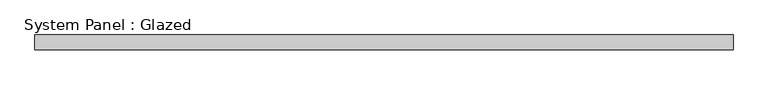
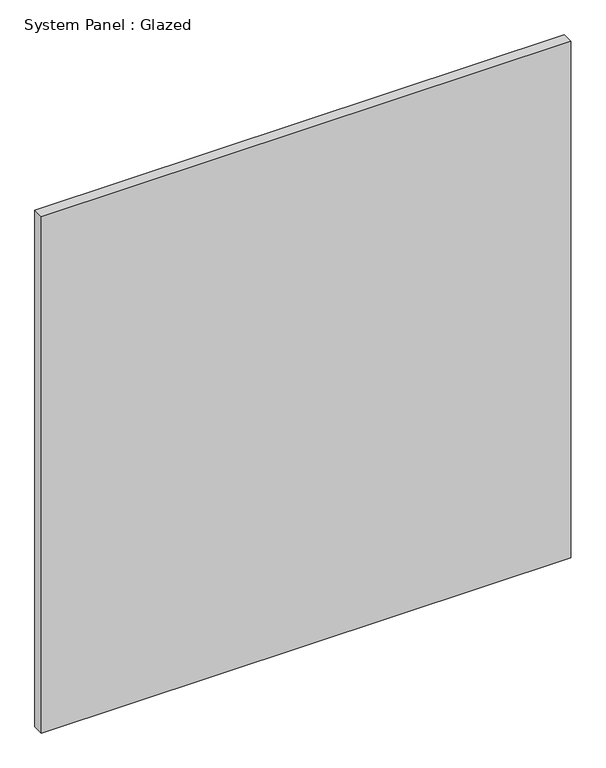
"""IFC4 building model written with IfcOpenShell, lengths in millimetres: plate geometry, System Panel : Glazed."""

from ifc_helpers import new_model, si_unit, origin, origin_with_axes, place, context, project, spatial, polyline, outline, extrude, source, transform, mapped, element, save


def system_panel_glazed_e4a816a2(model_context):
    return source(origin(), model_context, "Body", "SweptSolid", [
        extrude(outline(polyline([(591.0264963, 19.05), (-591.0264963, 19.05), (-591.0264963, 44.45), (591.0264963, 44.45), (591.0264963, 19.05)])), origin_with_axes(), (0.0, 0.0, 1.0), 1219.2),
    ])


if __name__ == "__main__":
    model = new_model("IFC4")
    model_context = context("Model", 3, world=origin())
    ifc_project = project(units=[si_unit("LENGTHUNIT", "METRE", prefix="MILLI")], contexts=[model_context])
    site = spatial("IfcSite", under=ifc_project)
    building = spatial("IfcBuilding", under=site)
    placement = place(None, origin())
    system_panel_glazed_shape = system_panel_glazed_e4a816a2(model_context)
    element("IfcPlate", 1, ObjectType="System Panel : Glazed", at=placement, inside=building, context=model_context, shape_type="MappedRepresentation", body=[
        mapped(system_panel_glazed_shape, transform((0.0, 0.0, 0.0), x_axis=(1.0, 0.0, 0.0), y_axis=(0.0, 1.0, 0.0), z_axis=(0.0, 0.0, 1.0))),
    ])
    save(model, "model.ifc")

# Revit data of these elements
# Type "System Panel : Glazed"
#   Construction Type Id = "GSP4R"
#   Analytic Construction = "1/8 in Pilkington single glazing"
#   Visual Light Transmittance = 0.9
#   Solar Heat Gain Coefficient = 0.86
#   Heat Transfer Coefficient (U) = 1.18115 BTU/(h·ft²·°F)
# Element 1 (IfcPlate, "System Panel : Glazed")
#   Materials on its faces: "Glass"
# Materials
#   "Glass": class "Glass", colour RGB 0 128 192, transparency 0.75, Description = "Soda Lime Glass", Cost = 0
